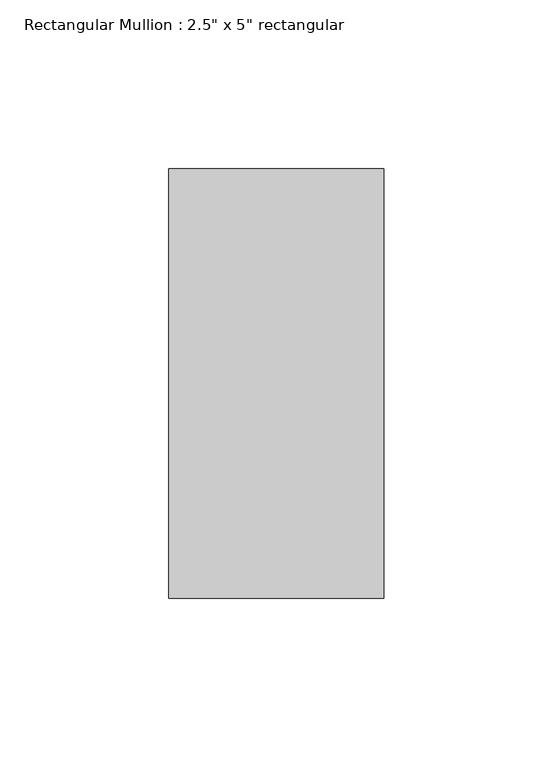
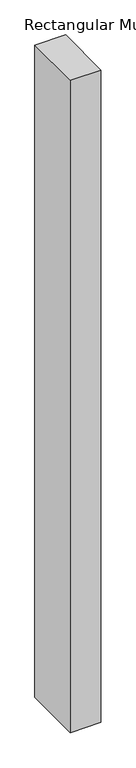
"""IFC4 building model written with IfcOpenShell, lengths in millimetres: member geometry."""

from ifc_helpers import new_model, si_unit, frame, origin, place, context, project, spatial, polyline, outline, extrude, source, transform, mapped, element, save


def member_04a79ac1(model_context):
    return source(origin(), model_context, "Body", "SweptSolid", [
        extrude(outline(polyline([(31.75, 63.5), (31.75, -63.5), (-31.75, -63.5), (-31.75, 63.5), (31.75, 63.5)])), frame((0.0, 0.0, -1431.017105), z_axis=(0.0, 0.0, 1.0), x_axis=(1.0, 0.0, 0.0)), (0.0, 0.0, 1.0), 1431.017105),
    ])


if __name__ == "__main__":
    model = new_model("IFC4")
    model_context = context("Model", 3, world=origin())
    ifc_project = project(units=[si_unit("LENGTHUNIT", "METRE", prefix="MILLI")], contexts=[model_context])
    site = spatial("IfcSite", under=ifc_project)
    building = spatial("IfcBuilding", under=site)
    placement = place(None, origin())
    member_shape = member_04a79ac1(model_context)
    element("IfcMember", 1, ObjectType="Rectangular Mullion : 2.5\" x 5\" rectangular", at=placement, inside=building, context=model_context, shape_type="MappedRepresentation", body=[
        mapped(member_shape, transform((0.0, 0.0, 0.0), x_axis=(1.0, 0.0, 0.0), y_axis=(0.0, 1.0, 0.0), z_axis=(0.0, 0.0, 1.0))),
    ])
    save(model, "model.ifc")

# Revit data of these elements
# Type "Rectangular Mullion : 2.5\" x 5\" rectangular"
#   built-in parameter 1007304 = 0.416667 (stored number, unit not read)
#   built-in parameter 1007301 = 0.104167 (stored number, unit not read)
#   built-in parameter 1007300 = 0.104167 (stored number, unit not read)
# Element 1 (IfcMember, "Rectangular Mullion : 2.5\" x 5\" rectangular")
#   Materials on its faces: "Aluminum"
# Materials
#   "Aluminum": class "Metal", colour RGB 247 247 247, transparency 0, Description = "Aluminum 6061", Cost = 0
